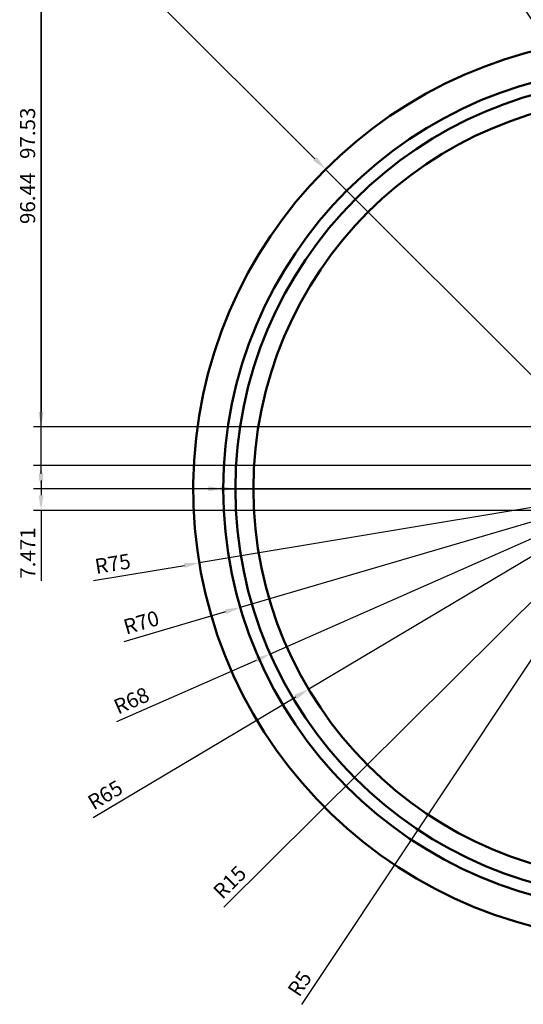
# Model space of a CAD drawing. Units: millimetres. Extents: x 1068 to 1546, y 1743 to 2032.
# Tile 1 of 9: x 1068 to 1152, y 1764 to 1928. Entities that reach past the tile are written whole.
import ezdxf

# ---------------------------------------------------------------- set-up
doc = ezdxf.new("R2010")
doc.units = ezdxf.units.MM
doc.layers.add('M-DIMS', color=2, linetype='Continuous', lineweight=25)
doc.layers.add('M-OUTL', color=7, linetype='Continuous', lineweight=50)
doc.styles.get("Standard").update_dxf_attribs({"font": 'arial.ttf'})
doc.dimstyles.new('ISO-25', dxfattribs={"dimtxt": 2.5, "dimasz": 2.5, "dimexe": 1.25, "dimexo": 0.625, "dimtad": 1, "dimtxsty": 'Standard', "dimcen": 2.5, "dimadec": 0, "dimazin": 0, "dimtfac": 1, "dimtmove": 0, "dimatfit": 3, "dimfxl": 1, "dimarcsym": 0})

# ---------------------------------------------------------------- blocks, each defined once
blk = doc.blocks.new('*D12')
at = {"layer": 'Defpoints', "color": 0, "transparency": 16777216}
for p in [(1172.23, 1849.76), (1169.46, 1845.6)]:
    blk.add_point(p, dxfattribs=at)
at = {"layer": 'M-DIMS', "color": 0, "lineweight": -2, "transparency": 16777216}
for p, q in [((1172.23, 1849.76), (1169.46, 1845.6)), ((1115.28, 1764.16), (1168.07, 1843.52))]:
    blk.add_line(p, q, dxfattribs=at)
at = {"layer": 'M-DIMS', "color": 0, "transparency": 16777216}
blk.add_solid([(1167.73, 1843.75), (1168.42, 1843.29), (1169.46, 1845.6)], dxfattribs=at)
at = {"layer": 'M-DIMS', "color": 0, "transparency": 16777216, "insert": (1115.17, 1767.42), "char_height": 2.5, "attachment_point": 5, "rotation": 56.3651}
blk.add_mtext('R5', dxfattribs=at)
blk = doc.blocks.new('*D13')
at = {"layer": 'Defpoints', "color": 0, "transparency": 16777216}
for p in [(1172.23, 1849.76), (1161.59, 1839.19)]:
    blk.add_point(p, dxfattribs=at)
at = {"layer": 'M-DIMS', "color": 0, "lineweight": -2, "transparency": 16777216}
for p, q in [((1172.23, 1849.76), (1161.59, 1839.19)), ((1102.29, 1780.3), (1159.81, 1837.43))]:
    blk.add_line(p, q, dxfattribs=at)
at = {"layer": 'M-DIMS', "color": 0, "transparency": 16777216}
blk.add_solid([(1159.52, 1837.73), (1160.11, 1837.13), (1161.59, 1839.19)], dxfattribs=at)
at = {"layer": 'M-DIMS', "color": 0, "transparency": 16777216, "insert": (1103.52, 1784.2), "char_height": 2.5, "attachment_point": 5, "rotation": 44.8055}
blk.add_mtext('R15', dxfattribs=at)
blk = doc.blocks.new('*D14')
at = {"layer": 'Defpoints', "color": 0, "transparency": 16777216}
for p in [(1172.23, 1849.76), (1116.4, 1816.48)]:
    blk.add_point(p, dxfattribs=at)
at = {"layer": 'M-DIMS', "color": 0, "lineweight": -2, "transparency": 16777216}
for p, q in [((1172.23, 1849.76), (1116.4, 1816.48)), ((1080.65, 1795.17), (1114.25, 1815.2))]:
    blk.add_line(p, q, dxfattribs=at)
at = {"layer": 'M-DIMS', "color": 0, "transparency": 16777216}
blk.add_solid([(1114.03, 1815.56), (1114.46, 1814.84), (1116.4, 1816.48)], dxfattribs=at)
at = {"layer": 'M-DIMS', "color": 0, "transparency": 16777216, "insert": (1082.79, 1798.66), "char_height": 2.5, "attachment_point": 5, "rotation": 30.7992}
blk.add_mtext('R65', dxfattribs=at)
blk = doc.blocks.new('*D15')
at = {"layer": 'Defpoints', "color": 0, "transparency": 16777216}
for p in [(1172.23, 1849.76), (1110.01, 1822.32)]:
    blk.add_point(p, dxfattribs=at)
at = {"layer": 'M-DIMS', "color": 0, "lineweight": -2, "transparency": 16777216}
for p, q in [((1172.23, 1849.76), (1110.01, 1822.32)), ((1084.58, 1811.1), (1107.72, 1821.31))]:
    blk.add_line(p, q, dxfattribs=at)
at = {"layer": 'M-DIMS', "color": 0, "transparency": 16777216}
blk.add_solid([(1107.55, 1821.69), (1107.89, 1820.93), (1110.01, 1822.32)], dxfattribs=at)
at = {"layer": 'M-DIMS', "color": 0, "transparency": 16777216, "insert": (1087.12, 1814.3), "char_height": 2.5, "attachment_point": 5, "rotation": 23.7993}
blk.add_mtext('R68', dxfattribs=at)
blk = doc.blocks.new('*D16')
at = {"layer": 'Defpoints', "color": 0, "transparency": 16777216}
for p in [(1172.23, 1849.76), (1105.05, 1830.07)]:
    blk.add_point(p, dxfattribs=at)
at = {"layer": 'M-DIMS', "color": 0, "lineweight": -2, "transparency": 16777216}
for p, q in [((1172.23, 1849.76), (1105.05, 1830.07)), ((1085.78, 1824.42), (1102.66, 1829.37))]:
    blk.add_line(p, q, dxfattribs=at)
at = {"layer": 'M-DIMS', "color": 0, "transparency": 16777216}
blk.add_solid([(1102.54, 1829.77), (1102.77, 1828.97), (1105.05, 1830.07)], dxfattribs=at)
at = {"layer": 'M-DIMS', "color": 0, "transparency": 16777216, "insert": (1088.71, 1827.26), "char_height": 2.5, "attachment_point": 5, "rotation": 16.3386}
blk.add_mtext('R70', dxfattribs=at)
blk = doc.blocks.new('*D17')
at = {"layer": 'Defpoints', "color": 0, "transparency": 16777216}
for p in [(1172.23, 1849.76), (1098.24, 1837.46)]:
    blk.add_point(p, dxfattribs=at)
at = {"layer": 'M-DIMS', "color": 0, "lineweight": -2, "transparency": 16777216}
for p, q in [((1172.23, 1849.76), (1098.24, 1837.46)), ((1080.67, 1834.54), (1095.78, 1837.05))]:
    blk.add_line(p, q, dxfattribs=at)
at = {"layer": 'M-DIMS', "color": 0, "transparency": 16777216}
blk.add_solid([(1095.71, 1837.46), (1095.85, 1836.64), (1098.24, 1837.46)], dxfattribs=at)
at = {"layer": 'M-DIMS', "color": 0, "transparency": 16777216, "insert": (1083.93, 1837), "char_height": 2.5, "attachment_point": 5, "rotation": 9.4427}
blk.add_mtext('R75', dxfattribs=at)
blk = doc.blocks.new('*D23')
at = {"layer": 'Defpoints', "color": 0, "transparency": 16777216}
for p in [(1170.51, 1998.5), (1125.92, 1968.44), (1270.79, 1849.76)]:
    blk.add_point(p, dxfattribs=at)
at = {"layer": 'M-DIMS', "color": 0, "lineweight": -2, "transparency": 16777216}
for p, q in [((1169.99, 1998.15), (1124.89, 1967.74)), ((1224.8, 1821.77), (1127.32, 1966.36)), ((1270.27, 1849.41), (1225.16, 1819))]:
    blk.add_line(p, q, dxfattribs=at)
at = {"layer": 'M-DIMS', "color": 0, "transparency": 16777216}
for points in [[(1127.67, 1966.6), (1126.98, 1966.13), (1125.92, 1968.44)], [(1225.15, 1822.01), (1224.45, 1821.54), (1226.2, 1819.7)]]:
    blk.add_solid(points, dxfattribs=at)
at = {"layer": 'M-DIMS', "color": 0, "transparency": 16777216, "insert": (1177.82, 1895.26), "char_height": 2.5, "attachment_point": 5, "rotation": 303.9872}
blk.add_mtext('179,38', dxfattribs=at)
blk = doc.blocks.new('*D28')
at = {"layer": 'Defpoints', "color": 0, "transparency": 16777216}
for p in [(1071.98, 1946.21), (1212.68, 1946.21), (1172.23, 1849.76)]:
    blk.add_point(p, dxfattribs=at)
at = {"layer": 'M-DIMS', "color": 0, "lineweight": -2, "transparency": 16777216}
for p, q in [((1212.06, 1946.21), (1070.73, 1946.21)), ((1071.98, 1852.26), (1071.98, 1943.71)), ((1171.6, 1849.76), (1070.73, 1849.76))]:
    blk.add_line(p, q, dxfattribs=at)
at = {"layer": 'M-DIMS', "color": 0, "transparency": 16777216}
for points in [[(1071.57, 1943.71), (1072.4, 1943.71), (1071.98, 1946.21)], [(1071.57, 1852.26), (1072.4, 1852.26), (1071.98, 1849.76)]]:
    blk.add_solid(points, dxfattribs=at)
at = {"layer": 'M-DIMS', "color": 0, "transparency": 16777216, "insert": (1070.08, 1897.98), "char_height": 2.5, "attachment_point": 5, "rotation": 90}
blk.add_mtext('96.44', dxfattribs=at)
blk = doc.blocks.new('*D46')
at = {"layer": 'Defpoints', "color": 0, "transparency": 16777216}
for p in [(1212.56, 1957.56), (1071.98, 1860.03), (1273.55, 1860.03)]:
    blk.add_point(p, dxfattribs=at)
at = {"layer": 'M-DIMS', "color": 0, "lineweight": -2, "transparency": 16777216}
for p, q in [((1211.93, 1957.56), (1070.73, 1957.56)), ((1071.98, 1955.06), (1071.98, 1862.53)), ((1272.92, 1860.03), (1070.73, 1860.03))]:
    blk.add_line(p, q, dxfattribs=at)
at = {"layer": 'M-DIMS', "color": 0, "transparency": 16777216}
for points in [[(1071.57, 1955.06), (1072.4, 1955.06), (1071.98, 1957.56)], [(1071.57, 1862.53), (1072.4, 1862.53), (1071.98, 1860.03)]]:
    blk.add_solid(points, dxfattribs=at)
at = {"layer": 'M-DIMS', "color": 0, "transparency": 16777216, "insert": (1070.08, 1908.79), "char_height": 2.5, "attachment_point": 5, "rotation": 90}
blk.add_mtext('97.53', dxfattribs=at)
blk = doc.blocks.new('*D50')
at = {"layer": 'Defpoints', "color": 0, "transparency": 16777216}
for p in [(1261.6, 1853.65), (1071.98, 1846.18), (1262.3, 1846.18)]:
    blk.add_point(p, dxfattribs=at)
at = {"layer": 'M-DIMS', "color": 0, "lineweight": -2, "transparency": 16777216}
for p, q in [((1260.97, 1853.65), (1070.73, 1853.65)), ((1071.98, 1851.15), (1071.98, 1848.68)), ((1261.67, 1846.18), (1070.73, 1846.18)), ((1071.98, 1846.18), (1071.98, 1834.5))]:
    blk.add_line(p, q, dxfattribs=at)
at = {"layer": 'M-DIMS', "color": 0, "transparency": 16777216}
for points in [[(1071.57, 1851.15), (1072.4, 1851.15), (1071.98, 1853.65)], [(1071.57, 1848.68), (1072.4, 1848.68), (1071.98, 1846.18)]]:
    blk.add_solid(points, dxfattribs=at)
at = {"layer": 'M-DIMS', "color": 0, "transparency": 16777216, "insert": (1070.1, 1839.09), "char_height": 2.5, "attachment_point": 5, "rotation": 90}
blk.add_mtext('7.471', dxfattribs=at)
blk = doc.blocks.new('*D57')
at = {"layer": 'Defpoints', "color": 0, "transparency": 16777216}
for p in [(1119.2, 1902.8), (1172.23, 1849.76)]:
    blk.add_point(p, dxfattribs=at)
at = {"layer": 'M-DIMS', "color": 0, "lineweight": -2, "transparency": 16777216}
for p, q in [((1084.82, 1937.18), (1117.43, 1904.57)), ((1172.23, 1849.76), (1119.2, 1902.8))]:
    blk.add_line(p, q, dxfattribs=at)
at = {"layer": 'M-DIMS', "color": 0, "transparency": 16777216}
blk.add_solid([(1117.73, 1904.86), (1117.14, 1904.27), (1119.2, 1902.8)], dxfattribs=at)
at = {"layer": 'M-DIMS', "color": 0, "transparency": 16777216, "insert": (1088.72, 1935.96), "char_height": 2.5, "attachment_point": 5, "rotation": 314.9948}
blk.add_mtext('R75', dxfattribs=at)
blk = doc.blocks.new('*D58')
at = {"layer": 'Defpoints', "color": 0, "transparency": 16777216}
for p in [(1102.23, 1849.76), (1242.23, 1849.76)]:
    blk.add_point(p, dxfattribs=at)
at = {"layer": 'M-DIMS', "color": 0, "lineweight": -2, "transparency": 16777216}
for p, q in [((1099.73, 1849.76), (1097.23, 1849.76)), ((1102.23, 1849.76), (1242.23, 1849.76)), ((1288.97, 1849.76), (1244.73, 1849.76))]:
    blk.add_line(p, q, dxfattribs=at)
at = {"layer": 'M-DIMS', "color": 0, "transparency": 16777216}
for points in [[(1099.73, 1850.18), (1099.73, 1849.35), (1102.23, 1849.76)], [(1244.73, 1850.18), (1244.73, 1849.35), (1242.23, 1849.76)]]:
    blk.add_solid(points, dxfattribs=at)
at = {"layer": 'M-DIMS', "color": 0, "transparency": 16777216, "insert": (1284.23, 1851.73), "char_height": 2.5, "attachment_point": 5, "rotation": 359.9997}
blk.add_mtext('∅140', dxfattribs=at)
blk = doc.blocks.new('*D59')
at = {"layer": 'Defpoints', "color": 0, "transparency": 16777216}
for p in [(1104.23, 1849.76), (1240.23, 1849.76)]:
    blk.add_point(p, dxfattribs=at)
at = {"layer": 'M-DIMS', "color": 0, "lineweight": -2, "transparency": 16777216}
for p, q in [((1101.73, 1849.76), (1099.23, 1849.76)), ((1104.23, 1849.76), (1240.23, 1849.76)), ((1285.77, 1849.76), (1242.73, 1849.76))]:
    blk.add_line(p, q, dxfattribs=at)
at = {"layer": 'M-DIMS', "color": 0, "transparency": 16777216}
for points in [[(1101.73, 1850.18), (1101.73, 1849.35), (1104.23, 1849.76)], [(1242.73, 1850.18), (1242.73, 1849.35), (1240.23, 1849.76)]]:
    blk.add_solid(points, dxfattribs=at)
at = {"layer": 'M-DIMS', "color": 0, "transparency": 16777216, "insert": (1281.03, 1851.73), "char_height": 2.5, "attachment_point": 5, "rotation": 359.9997}
blk.add_mtext('∅136', dxfattribs=at)

msp = doc.modelspace()

# ---------------------------------------------------------------- linework, layer by layer
at = {"layer": 'M-OUTL'}
for radius in [70, 68, 65]:
    msp.add_circle((1172.2281, 1849.7623), radius, dxfattribs=at)
msp.add_arc((1172.2281, 1849.7623), 75, 2.898254, 355.67622, dxfattribs=at)

# ---------------------------------------------------------------- dimensions: what is measured, and where the dimension line sits
at = {"layer": 'M-DIMS'}
dim = msp.add_aligned_dim(p1=(1270.787, 1849.7623), p2=(1170.5128, 1998.4966), distance=53.7765, dimstyle='ISO-25', override={"dimclrd": 0, "dimclre": 0, "dimclrt": 0}, dxfattribs=at)
dim.commit()
dim.dimension.update_dxf_attribs({"geometry": '*D23', "text_midpoint": (1177.8244, 1895.2572)})
for base, p1, p2, override, picture, middle in [((1071.9839, 1860.0259), (1212.5594, 1957.5607), (1273.5484, 1860.0259), {"dimdec": 2, "dimlfac": 1, "dimrnd": 0, "dimzin": 0, "dimdsep": 46, "dimlunit": 2}, '*D46', (1070.0816, 1908.7933)), ((1071.9839, 1946.2068), (1172.2281, 1849.7623), (1212.6811, 1946.2068), {"dimdec": 2, "dimlfac": 1, "dimrnd": 0, "dimzin": 0, "dimdsep": 46, "dimlunit": 2}, '*D28', (1070.0825, 1897.9845)), ((1071.9839, 1846.1816), (1261.5989, 1853.653), (1262.2997, 1846.1816), {"dimdec": 3, "dimlfac": 1, "dimrnd": 0, "dimzin": 0, "dimdsep": 46, "dimlunit": 2}, '*D50', (1070.1038, 1839.09))]:
    dim = msp.add_linear_dim(base=base, p1=p1, p2=p2, angle=90, dimstyle='ISO-25', override=override, dxfattribs=at)
    dim.commit()
    dim.dimension.update_dxf_attribs({"geometry": picture, "text_midpoint": middle})
for mpoint, override, picture, middle in [((1119.1999, 1902.8001), {"dimdec": 0, "dimlfac": 1, "dimrnd": 0, "dimzin": 0, "dimdsep": 46, "dimlunit": 2}, '*D57', (1087.383, 1934.6228)), ((1116.3952, 1816.4804), {"dimclrd": 0, "dimclre": 0, "dimclrt": 0}, '*D14', (1083.764, 1797.0289)), ((1098.2444, 1837.4577), {"dimclrd": 0, "dimclre": 0, "dimclrt": 0}, '*D17', (1084.2443, 1835.1292)), ((1110.0105, 1822.322), {"dimclrd": 0, "dimclre": 0, "dimclrt": 0}, '*D15', (1087.8824, 1812.5626)), ((1105.055, 1830.0704), {"dimclrd": 0, "dimclre": 0, "dimclrt": 0}, '*D16', (1089.2466, 1825.4362)), ((1161.5856, 1839.1918), {"dimclrd": 0, "dimclre": 0, "dimclrt": 0}, '*D13', (1104.8597, 1782.8497)), ((1169.4586, 1845.5994), {"dimclrd": 0, "dimclre": 0, "dimclrt": 0}, '*D12', (1116.7499, 1766.3712))]:
    dim = msp.add_radius_dim(center=(1172.2281, 1849.7623), mpoint=mpoint, dimstyle='ISO-25', override=override, dxfattribs=at)
    dim.commit()
    dim.dimension.update_dxf_attribs({"geometry": picture, "text_midpoint": middle, "dimtype": 164})
for p1, p2, picture, middle in [((1102.2281, 1849.7627), (1242.2281, 1849.762), '*D58', (1284.2281, 1849.7618)), ((1104.2281, 1849.7627), (1240.2281, 1849.762), '*D59', (1281.0281, 1849.7618))]:
    dim = msp.add_diameter_dim_2p(p1=p1, p2=p2, dimstyle='ISO-25', override={"dimdec": 0, "dimlfac": 1, "dimrnd": 0, "dimzin": 0, "dimdsep": 46, "dimlunit": 2}, dxfattribs=at)
    dim.commit()
    dim.dimension.update_dxf_attribs({"geometry": picture, "text_midpoint": middle, "dimtype": 163})

doc.saveas('drawing.dxf')
